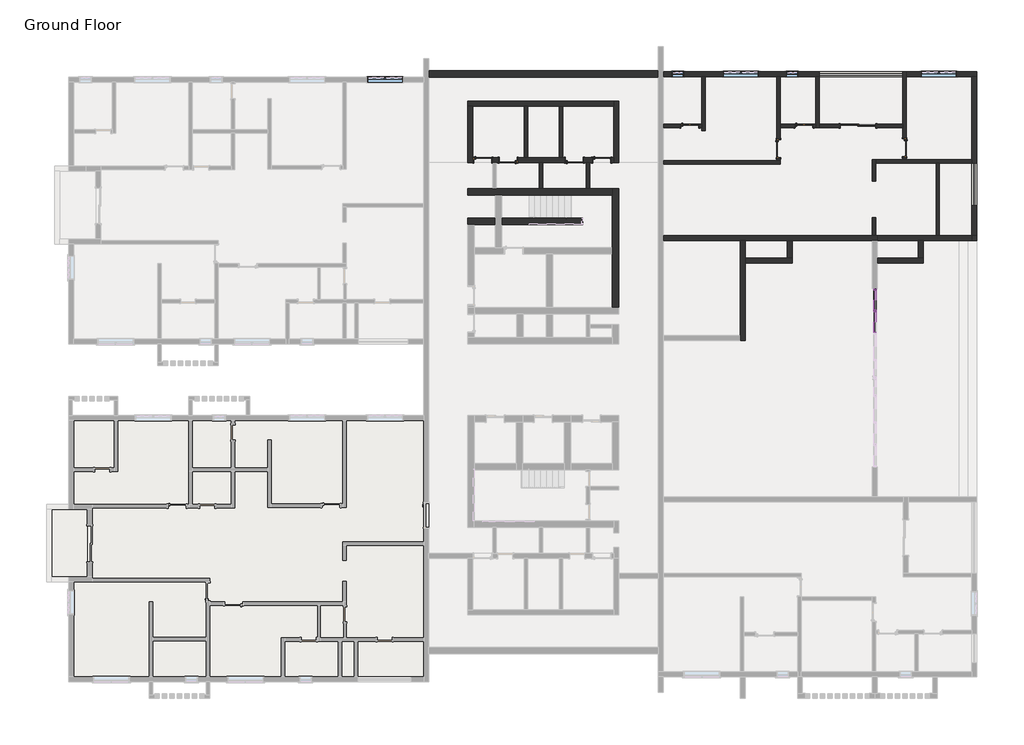
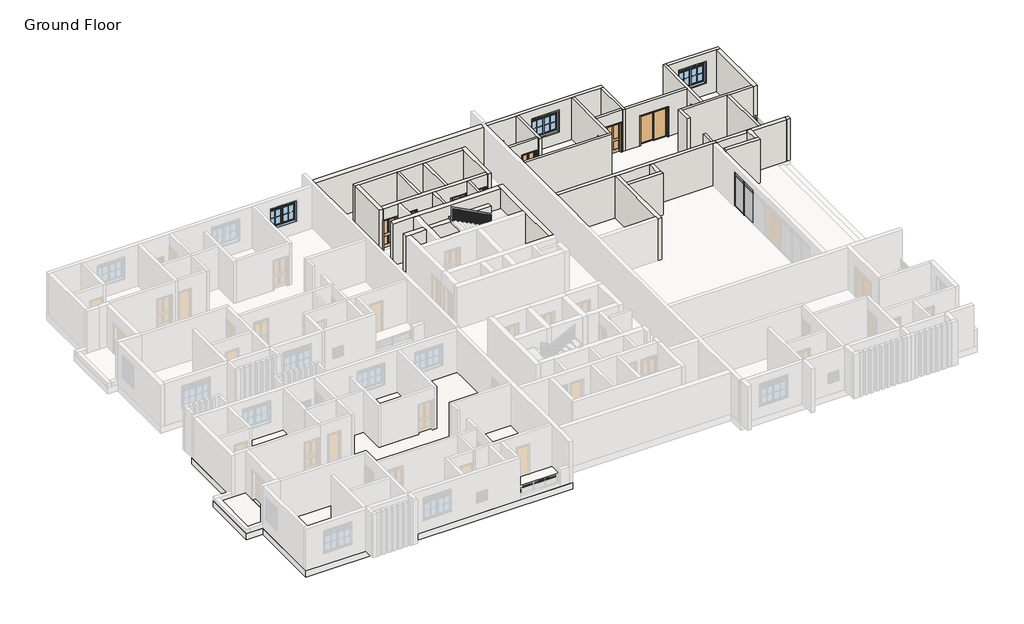
# One storey, part 5 of 9: 38 walls, 9 doors, 9 members, 5 windows, 4 plates, 2 slabs.
# Revit data of these elements (continued)
# Elements 59, 62 (IfcWall, "9\" EXTERIOR WALL")
#   Top Offset = 0' - 0"
#   Base Offset = 0' - 0"
#   Unconnected Height = 1' - 0"
#   wall height = 1' - 0"
#   Phase Created = New Construction
#   Base Constraint = Ground Floor
#   Materials on its faces: "Default Wall", "0 Cream"
# Element 61 (IfcWall, "9\" EXTERIOR WALL")
#   Top Offset = 0' - 0"
#   Base Offset = 0' - 0"
#   Unconnected Height = 4' - 0"
#   wall height = 4' - 0"
#   Phase Created = New Construction
#   Base Constraint = Ground Floor
#   Materials on its faces: "Default Wall", "0 Cream"
# Element 63 (IfcWindow, "Window-Casement-Double-Awning-Double : 6' x 5'")
#   Mark = "12"
#   Window Inset = 0' - 0"
#   Interior Wall Closure = 0' - 2 1/4"
#   Frame Extension = 0' - 0 1/4"
#   Exterior Wall Closure = 0' - 1 1/4"
#   Interior Trim Visibility = yes
#   Exterior Trim Visibility = yes
#   Phase Created = New Construction
#   Materials on its faces: "Wood - Stained", "Glass", "Clad - White"
# Element 64 (IfcWindow, "Window-Casement-Double-Awning-Double : 6' x 5'")
#   Mark = "22"
#   Window Inset = 0' - 0"
#   Interior Wall Closure = 0' - 2 1/4"
#   Frame Extension = 0' - 0 1/4"
#   Exterior Wall Closure = 0' - 1 1/4"
#   Interior Trim Visibility = yes
#   Exterior Trim Visibility = yes
#   Phase Created = New Construction
#   Materials on its faces: "Wood - Stained", "Glass", "Clad - White"
# Element 65 (IfcWindow, "Window-Casement-Double-Awning-Double : 6' x 5'")
#   Mark = "23"
#   Window Inset = 0' - 0"
#   Interior Wall Closure = 0' - 2 1/4"
#   Frame Extension = 0' - 0 1/4"
#   Exterior Wall Closure = 0' - 1 1/4"
#   Interior Trim Visibility = yes
#   Exterior Trim Visibility = yes
#   Phase Created = New Construction
#   Materials on its faces: "Wood - Stained", "Glass", "Clad - White"
# Element 66 (IfcWindow, "Window-Double-Hung")
#   Mark = "24"
#   Window Inset = 0' - 0"
#   Interior Wall Closure = 0' - 1 1/2"
#   Frame Extension = 0' - 1 1/4"
#   Exterior Wall Closure = 0' - 0 1/2"
#   Interior Trim Visibility = yes
#   Indicator Visibility = yes
#   Exterior Trim Visibility = yes
#   Phase Created = New Construction
#   Materials on its faces: "Wood - Stained", "Glass", "Clad - White"
# Element 67 (IfcWindow, "Window-Double-Hung")
#   Mark = "25"
#   Window Inset = 0' - 0"
#   Interior Wall Closure = 0' - 1 1/2"
#   Frame Extension = 0' - 1 1/4"
#   Exterior Wall Closure = 0' - 0 1/2"
#   Interior Trim Visibility = yes
#   Indicator Visibility = yes
#   Exterior Trim Visibility = yes
#   Phase Created = New Construction
#   Materials on its faces: "Wood - Stained", "Glass", "Clad - White"
# Materials
#   "Glass": class "Glass", colour RGB 0 128 192, transparency 0.75, Description = "Soda Lime Glass", Cost = 0
#   "Wood - Birch - Solid Stained Light Low Gloss": class "Wood", colour RGB 210 159 95, transparency 0, Cost = 0
#   "Paint - Sienna": colour RGB 118 70 51, transparency 0, Cost = 0
#   "Cherry": class "Wood", colour RGB 226 177 128, transparency 0, Description = "Prunus Serotina", Cost = 0
#   "Aluminum": class "Metal", colour RGB 247 247 247, transparency 0, Description = "Aluminum 6061", Cost = 0
#   "0 deck(1)": class "Generic", colour RGB 120 120 120, transparency 0, Cost = 0
#   "0 cream Floor": class "Generic", colour RGB 120 120 120, transparency 0, Cost = 0
#   "0 Cream": class "Generic", colour RGB 120 120 120, transparency 0, Cost = 0
#   "Wood - Stained": class "Wood", colour RGB 224 178 126, transparency 0, Cost = 0
#   "Clad - White": class "Wood", colour RGB 242 242 238, transparency 0, Cost = 0
#   "0 olive green": class "Generic", colour RGB 120 120 120, transparency 0, Cost = 0
#   "Default Wall": colour RGB 128 128 128, transparency 0, Cost = 0
